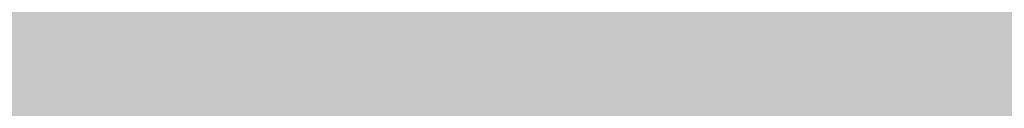
# Model space of a CAD drawing. Units: feet. Extents: x 3168 to 4724, y 827 to 1477.
# Tile 195 of 256: x 3316.07 to 3333.46, y 1096.78 to 1098.34. Entities that reach past the tile are written whole.
import ezdxf

# ---------------------------------------------------------------- set-up
doc = ezdxf.new("R2010")
doc.units = ezdxf.units.FT
doc.layers.add('A-ELEV-PATT', color=8, linetype='Continuous', lineweight=13)

msp = doc.modelspace()

# ---------------------------------------------------------------- hatches: boundary and pattern name
at = {"layer": 'A-ELEV-PATT'}
h = msp.add_hatch(color=256, dxfattribs=at)
h.dxf.hatch_style = 1
edge = h.paths.add_edge_path()
edge.add_ellipse((3552.906, 979.22), major_axis=(36.745, 0), ratio=0.484848, start_angle=0, end_angle=360)
edge = h.paths.add_edge_path()
edge.add_ellipse((3559.892, 929.252), major_axis=(36.745, 0), ratio=0.484848, start_angle=0, end_angle=360)
edge = h.paths.add_edge_path()
edge.add_line((3299.317, 1198.606), (3479.917, 1198.606))
edge.add_line((3479.917, 1198.606), (3479.917, 1209.869))
edge.add_spline(control_points=[(3479.917, 1209.869), (3464.301, 1209.869), (3448.686, 1209.869), (3410.949, 1209.869), (3388.828, 1209.869), (3355.647, 1209.869), (3344.586, 1209.869), (3327.996, 1209.869), (3322.466, 1209.869), (3314.17, 1209.869), (3311.405, 1209.869), (3307.257, 1209.869), (3305.875, 1209.869), (3303.801, 1209.869), (3303.11, 1209.869), (3302.073, 1209.869), (3301.727, 1209.869), (3301.209, 1209.869), (3301.036, 1209.869), (3300.777, 1209.869), (3300.69, 1209.869), (3300.561, 1209.869), (3300.517, 1209.869), (3300.453, 1209.869), (3300.431, 1209.869), (3300.399, 1209.869), (3300.388, 1209.869), (3300.366, 1209.869), (3300.346, 1209.869), (3300.346, 1209.869), (3300.346, 1209.869), (3300.343, 1209.869), (3300.341, 1209.869), (3300.338, 1209.869), (3300.337, 1209.869), (3300.334, 1209.869), (3300.332, 1209.869), (3300.326, 1209.869), (3300.321, 1209.869), (3300.311, 1209.869), (3300.306, 1209.869), (3300.291, 1209.869), (3300.28, 1209.869), (3300.232, 1209.869), (3300.195, 1209.869), (3299.951, 1209.871), (3299.745, 1209.874), (3299.437, 1209.883), (3299.334, 1209.887), (3299.181, 1209.893), (3299.13, 1209.895), (3298.652, 1209.917), (3298.229, 1209.946), (3297.602, 1210.002), (3297.393, 1210.023), (3297.083, 1210.058), (3296.979, 1210.07), (3296.293, 1210.155), (3295.718, 1210.243), (3294.869, 1210.399), (3294.588, 1210.454), (3294.169, 1210.543), (3294.03, 1210.574), (3291.707, 1211.101), (3289.654, 1211.813), (3285.776, 1213.564), (3283.951, 1214.603), (3280.512, 1216.98), (3278.897, 1218.318), (3276.38, 1220.829), (3275.416, 1221.918), (3274.039, 1223.708), (3273.581, 1224.35), (3273.143, 1225.016)], knot_values=[39.119033, 39.119033, 39.119033, 39.119033, 39.286353, 39.286353, 39.523379, 39.523379, 39.641892, 39.641892, 39.701148, 39.701148, 39.730777, 39.730777, 39.745591, 39.745591, 39.752998, 39.752998, 39.756701, 39.756701, 39.758553, 39.758553, 39.759479, 39.759479, 39.759942, 39.759942, 39.760173, 39.760173, 39.760289, 39.760289, 39.760405, 39.760405, 39.760463, 39.760463, 39.763389, 39.763389, 39.764851, 39.764851, 39.767304, 39.767304, 39.773825, 39.773825, 39.78057, 39.78057, 39.79477, 39.79477, 39.845194, 39.845194, 40.126715, 40.126715, 40.267476, 40.267476, 40.337856, 40.337856, 40.927023, 40.927023, 41.221606, 41.221606, 41.368898, 41.368898, 42.202622, 42.202622, 42.619485, 42.619485, 42.827916, 42.827916, 46.118323, 46.118323, 49.408731, 49.408731, 52.699139, 52.699139, 54.927489, 54.927489, 56.104228, 56.104228, 56.104228, 56.104228], weights=[1, 1, 1, 1, 1, 1, 1, 1, 1, 1, 1, 1, 1, 1, 1, 1, 1, 1, 1, 1, 1, 1, 1, 1, 1, 1, 1, 1, 1, 1, 1, 1, 1, 1, 1, 1, 1, 1, 1, 1, 1, 1, 1, 1, 1, 1, 1, 1, 1, 1, 1, 1, 1, 1, 1, 1, 1, 1, 1, 1, 1, 1, 1, 1, 1, 1, 1, 1, 1, 1, 1, 1, 1, 1], degree=3, periodic=0)
edge.add_line((3273.143, 1225.016), (3273.143, 1099.016))
edge.add_line((3273.143, 1099.016), (3299.317, 1099.016))
edge.add_line((3299.317, 1099.016), (3299.317, 1198.606))
edge = h.paths.add_edge_path()
edge.add_line((3304.758, 1324.158), (3479.917, 1324.158))
edge.add_line((3479.917, 1324.158), (3479.917, 1335.715))
edge.add_line((3479.917, 1335.715), (3269.162, 1335.715))
edge.add_spline(control_points=[(3269.162, 1335.715), (3264.024, 1335.715), (3258.364, 1328.958), (3259.264, 1323.9)], knot_values=[0, 0, 0, 0, 15.412191, 15.412191, 15.412191, 15.412191], degree=3, periodic=0)
edge.add_line((3259.264, 1323.9), (3265.517, 1288.769))
edge.add_line((3265.517, 1288.769), (3275.265, 1261.546))
edge.add_line((3275.265, 1261.546), (3304.758, 1261.546))
edge.add_line((3304.758, 1261.546), (3304.758, 1324.158))
h = msp.add_hatch(color=256, dxfattribs=at)
h.dxf.hatch_style = 1
h.paths.add_polyline_path([(3384.525, 1099.016), (3335.029, 1099.016), (3299.317, 1099.016), (3273.143, 1099.016), (3217.565, 1099.016), (3168.069, 827.116), (3335.029, 827.116)])

doc.saveas('drawing.dxf')
